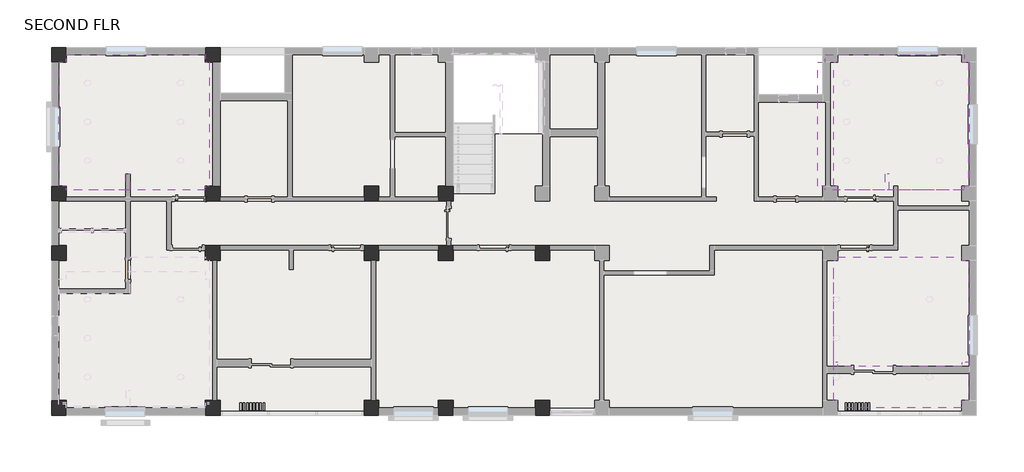
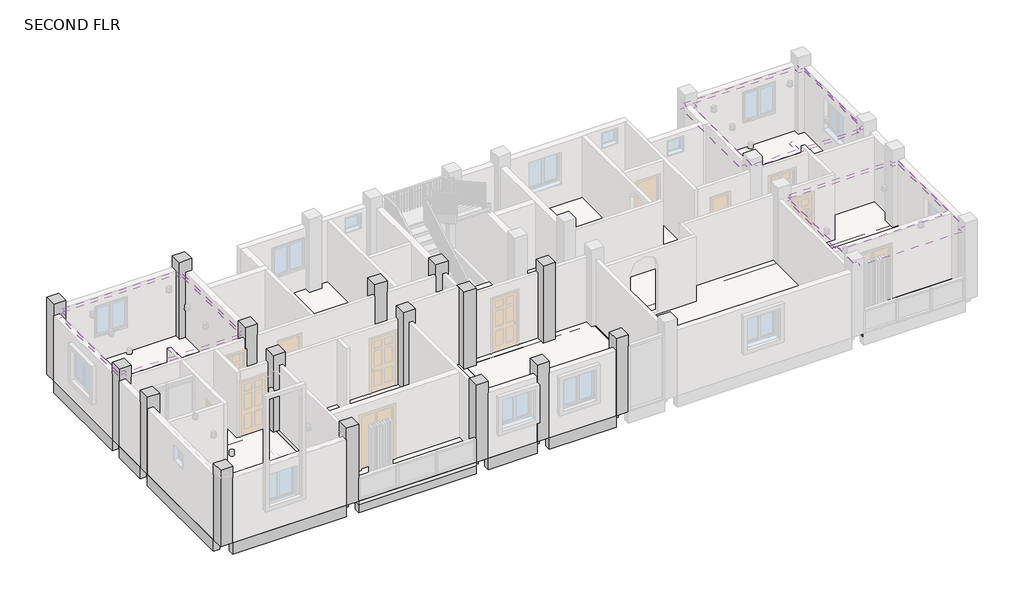
# One storey, part 3 of 5: 23 beams, 16 columns, 6 coverings, 3 slabs.
"""IFC4 building model written with IfcOpenShell, lengths in millimetres."""

from ifc_helpers import new_model, si_unit, point, frame, frame_2d, origin, place, context, project, spatial, polyline, circle_curve, trimmed, segment, composite_curve, outline, extrude, element, save

model = new_model("IFC4")

# Units and contexts
model_context = context("Model", 3, world=origin())
ifc_project = project(units=[si_unit("LENGTHUNIT", "METRE", prefix="MILLI")], contexts=[model_context])

# Site, building, storey
site = spatial("IfcSite", under=ifc_project)
building = spatial("IfcBuilding", under=site)
storey = spatial("IfcBuildingStorey", under=building, Name="SECOND FLR", Elevation=6400.8)

# Beams
placement = place(None, origin())
element("IfcBeam", 1, ObjectType="Concrete-Rectangular Beam : 9\" X 18\" BEAM", at=placement, inside=storey, context=model_context, shape_type="SweptSolid", body=[
    extrude(outline(polyline([(-10649.5456086, -10887.8679047), (-10649.5456086, -11116.4679047), (-14916.7456086, -11116.4679047), (-14916.7456086, -10887.8679047), (-10649.5456086, -10887.8679047)])), frame((0.0, 0.0, 5943.6), z_axis=(0.0, 0.0, 1.0), x_axis=(1.0, 0.0, 0.0)), (0.0, 0.0, 1.0), 457.2),
])
element("IfcBeam", 2, ObjectType="Concrete-Rectangular Beam : 9\" X 18\" BEAM", at=placement, inside=storey, context=model_context, shape_type="SweptSolid", body=[
    extrude(outline(polyline([(-5772.7456086, -10887.8679047), (-5772.7456086, -11116.4679047), (-10192.3456086, -11116.4679047), (-10192.3456086, -10887.8679047), (-5772.7456086, -10887.8679047)])), frame((0.0, 0.0, 5943.6), z_axis=(0.0, 0.0, 1.0), x_axis=(1.0, 0.0, 0.0)), (0.0, 0.0, 1.0), 457.2),
])
element("IfcBeam", 3, ObjectType="Concrete-Rectangular Beam : 9\" X 18\" BEAM", at=placement, inside=storey, context=model_context, shape_type="SweptSolid", body=[
    extrude(outline(polyline([(-3486.7456086, -10887.8679047), (-3486.7456086, -11116.4679047), (-5315.5456086, -11116.4679047), (-5315.5456086, -10887.8679047), (-3486.7456086, -10887.8679047)])), frame((0.0, 0.0, 5943.6), z_axis=(0.0, 0.0, 1.0), x_axis=(1.0, 0.0, 0.0)), (0.0, 0.0, 1.0), 457.2),
])
element("IfcBeam", 4, ObjectType="Concrete-Rectangular Beam : 9\" X 18\" BEAM", at=placement, inside=storey, context=model_context, shape_type="SweptSolid", body=[
    extrude(outline(polyline([(-518.4083398, -10887.8679047), (-518.4083398, -11116.4679047), (-3029.5456086, -11116.4679047), (-3029.5456086, -10887.8679047), (-518.4083398, -10887.8679047)])), frame((0.0, 0.0, 5943.6), z_axis=(0.0, 0.0, 1.0), x_axis=(1.0, 0.0, 0.0)), (0.0, 0.0, 1.0), 457.2),
])
element("IfcBeam", 5, ObjectType="Concrete-Rectangular Beam : 9\" X 18\" BEAM", at=placement, inside=storey, context=model_context, shape_type="SweptSolid", body=[
    extrude(outline(polyline([(-15145.3456086, -4072.3794704), (-15373.9456086, -4072.3794704), (-15373.9456086, -262.3794704), (-15145.3456086, -262.3794704), (-15145.3456086, -4072.3794704)])), frame((0.0, 0.0, 5943.6), z_axis=(0.0, 0.0, 1.0), x_axis=(1.0, 0.0, 0.0)), (0.0, 0.0, 1.0), 457.2),
])
element("IfcBeam", 6, ObjectType="Concrete-Rectangular Beam : 9\" X 18\" BEAM", at=placement, inside=storey, context=model_context, shape_type="SweptSolid", body=[
    extrude(outline(polyline([(-15145.3456086, -5901.1794704), (-15373.9456086, -5901.1794704), (-15373.9456086, -4529.5794704), (-15145.3456086, -4529.5794704), (-15145.3456086, -5901.1794704)])), frame((0.0, 0.0, 5943.6), z_axis=(0.0, 0.0, 1.0), x_axis=(1.0, 0.0, 0.0)), (0.0, 0.0, 1.0), 457.2),
])
element("IfcBeam", 7, ObjectType="Concrete-Rectangular Beam : 9\" X 18\" BEAM", at=placement, inside=storey, context=model_context, shape_type="SweptSolid", body=[
    extrude(outline(polyline([(-15145.3456086, -10659.2679047), (-15373.9456086, -10659.2679047), (-15373.9456086, -6358.3794704), (-15145.3456086, -6358.3794704), (-15145.3456086, -10659.2679047)])), frame((0.0, 0.0, 5943.6), z_axis=(0.0, 0.0, 1.0), x_axis=(1.0, 0.0, 0.0)), (0.0, 0.0, 1.0), 457.2),
])
element("IfcBeam", 8, ObjectType="Concrete-Rectangular Beam : 9\" X 18\" BEAM", at=placement, inside=storey, context=model_context, shape_type="SweptSolid", body=[
    extrude(outline(polyline([(-10649.5456086, -4186.6794704), (-10649.5456086, -4415.2794704), (-14916.7456086, -4415.2794704), (-14916.7456086, -4186.6794704), (-10649.5456086, -4186.6794704)])), frame((0.0, 0.0, 5943.6), z_axis=(0.0, 0.0, 1.0), x_axis=(1.0, 0.0, 0.0)), (0.0, 0.0, 1.0), 457.2),
])
element("IfcBeam", 9, ObjectType="Concrete-Rectangular Beam : 9\" X 18\" BEAM", at=placement, inside=storey, context=model_context, shape_type="SweptSolid", body=[
    extrude(outline(polyline([(-5772.7456086, -4186.6794704), (-5772.7456086, -4415.2794704), (-10192.3456086, -4415.2794704), (-10192.3456086, -4186.6794704), (-5772.7456086, -4186.6794704)])), frame((0.0, 0.0, 5943.6), z_axis=(0.0, 0.0, 1.0), x_axis=(1.0, 0.0, 0.0)), (0.0, 0.0, 1.0), 457.2),
])
element("IfcBeam", 10, ObjectType="Concrete-Rectangular Beam : 9\" X 18\" BEAM", at=placement, inside=storey, context=model_context, shape_type="SweptSolid", body=[
    extrude(outline(polyline([(-3486.7456086, -4186.6794704), (-3486.7456086, -4415.2794704), (-5315.5456086, -4415.2794704), (-5315.5456086, -4186.6794704), (-3486.7456086, -4186.6794704)])), frame((0.0, 0.0, 5943.6), z_axis=(0.0, 0.0, 1.0), x_axis=(1.0, 0.0, 0.0)), (0.0, 0.0, 1.0), 457.2),
])
element("IfcBeam", 11, ObjectType="Concrete-Rectangular Beam : 9\" X 18\" BEAM", at=placement, inside=storey, context=model_context, shape_type="SweptSolid", body=[
    extrude(outline(polyline([(-10306.6456086, -4072.3794704), (-10535.2456086, -4072.3794704), (-10535.2456086, -262.3794704), (-10306.6456086, -262.3794704), (-10306.6456086, -4072.3794704)])), frame((0.0, 0.0, 5943.6), z_axis=(0.0, 0.0, 1.0), x_axis=(1.0, 0.0, 0.0)), (0.0, 0.0, 1.0), 457.2),
])
element("IfcBeam", 12, ObjectType="Concrete-Rectangular Beam : 9\" X 18\" BEAM", at=placement, inside=storey, context=model_context, shape_type="SweptSolid", body=[
    extrude(outline(polyline([(-10649.5456086, -6015.4794704), (-10649.5456086, -6244.0794704), (-14916.7456086, -6244.0794704), (-14916.7456086, -6015.4794704), (-10649.5456086, -6015.4794704)])), frame((0.0, 0.0, 5943.6), z_axis=(0.0, 0.0, 1.0), x_axis=(1.0, 0.0, 0.0)), (0.0, 0.0, 1.0), 457.2),
])
element("IfcBeam", 13, ObjectType="Concrete-Rectangular Beam : 9\" X 18\" BEAM", at=placement, inside=storey, context=model_context, shape_type="SweptSolid", body=[
    extrude(outline(polyline([(-5772.7456086, -6015.4794704), (-5772.7456086, -6244.0794704), (-10192.3456086, -6244.0794704), (-10192.3456086, -6015.4794704), (-5772.7456086, -6015.4794704)])), frame((0.0, 0.0, 5943.6), z_axis=(0.0, 0.0, 1.0), x_axis=(1.0, 0.0, 0.0)), (0.0, 0.0, 1.0), 457.2),
])
element("IfcBeam", 14, ObjectType="Concrete-Rectangular Beam : 9\" X 18\" BEAM", at=placement, inside=storey, context=model_context, shape_type="SweptSolid", body=[
    extrude(outline(polyline([(-3486.7456086, -6015.4794704), (-3486.7456086, -6244.0794704), (-5315.5456086, -6244.0794704), (-5315.5456086, -6015.4794704), (-3486.7456086, -6015.4794704)])), frame((0.0, 0.0, 5943.6), z_axis=(0.0, 0.0, 1.0), x_axis=(1.0, 0.0, 0.0)), (0.0, 0.0, 1.0), 457.2),
])
element("IfcBeam", 15, ObjectType="Concrete-Rectangular Beam : 9\" X 18\" BEAM", at=placement, inside=storey, context=model_context, shape_type="SweptSolid", body=[
    extrude(outline(polyline([(-3029.5456086, -6244.0794704), (-3029.5456086, -6015.4794704), (-518.4083398, -6015.4794704), (-518.4083398, -6244.0794704), (-3029.5456086, -6244.0794704)])), frame((0.0, 0.0, 5943.6), z_axis=(0.0, 0.0, 1.0), x_axis=(1.0, 0.0, 0.0)), (0.0, 0.0, 1.0), 457.2),
])
element("IfcBeam", 16, ObjectType="Concrete-Rectangular Beam : 9\" X 18\" BEAM", at=placement, inside=storey, context=model_context, shape_type="SweptSolid", body=[
    extrude(outline(polyline([(-10535.2456086, -6358.3794704), (-10306.6456086, -6358.3794704), (-10306.6456086, -10659.2679047), (-10535.2456086, -10659.2679047), (-10535.2456086, -6358.3794704)])), frame((0.0, 0.0, 5943.6), z_axis=(0.0, 0.0, 1.0), x_axis=(1.0, 0.0, 0.0)), (0.0, 0.0, 1.0), 457.2),
])
element("IfcBeam", 17, ObjectType="Concrete-Rectangular Beam : 9\" X 18\" BEAM", at=placement, inside=storey, context=model_context, shape_type="SweptSolid", body=[
    extrude(outline(polyline([(-5658.4456086, -6358.3794704), (-5429.8456086, -6358.3794704), (-5429.8456086, -10659.2679047), (-5658.4456086, -10659.2679047), (-5658.4456086, -6358.3794704)])), frame((0.0, 0.0, 5943.6), z_axis=(0.0, 0.0, 1.0), x_axis=(1.0, 0.0, 0.0)), (0.0, 0.0, 1.0), 457.2),
])
element("IfcBeam", 18, ObjectType="Concrete-Rectangular Beam : 9\" X 18\" BEAM", at=placement, inside=storey, context=model_context, shape_type="SweptSolid", body=[
    extrude(outline(polyline([(-3372.4456086, -6358.3794704), (-3143.8456086, -6358.3794704), (-3143.8456086, -10659.2679047), (-3372.4456086, -10659.2679047), (-3372.4456086, -6358.3794704)])), frame((0.0, 0.0, 5943.6), z_axis=(0.0, 0.0, 1.0), x_axis=(1.0, 0.0, 0.0)), (0.0, 0.0, 1.0), 457.2),
])
element("IfcBeam", 19, ObjectType="Concrete-Rectangular Beam : 9\" X 18\" BEAM", at=placement, inside=storey, context=model_context, shape_type="SweptSolid", body=[
    extrude(outline(polyline([(-404.1083398, -6358.3794704), (-175.5083398, -6358.3794704), (-175.5083398, -10659.2679047), (-404.1083398, -10659.2679047), (-404.1083398, -6358.3794704)])), frame((0.0, 0.0, 5943.6), z_axis=(0.0, 0.0, 1.0), x_axis=(1.0, 0.0, 0.0)), (0.0, 0.0, 1.0), 457.2),
])
element("IfcBeam", 20, ObjectType="Concrete-Rectangular Beam : 9\" X 18\" BEAM", at=placement, inside=storey, context=model_context, shape_type="SweptSolid", body=[
    extrude(outline(polyline([(-404.1083398, -4529.5794704), (-175.5083398, -4529.5794704), (-175.5083398, -5901.1794704), (-404.1083398, -5901.1794704), (-404.1083398, -4529.5794704)])), frame((0.0, 0.0, 5943.6), z_axis=(0.0, 0.0, 1.0), x_axis=(1.0, 0.0, 0.0)), (0.0, 0.0, 1.0), 457.2),
])
element("IfcBeam", 21, ObjectType="Concrete-Rectangular Beam : 9\" X 18\" BEAM", at=placement, inside=storey, context=model_context, shape_type="SweptSolid", body=[
    extrude(outline(polyline([(-3143.8456086, -5901.1794704), (-3372.4456086, -5901.1794704), (-3372.4456086, -4529.5794704), (-3143.8456086, -4529.5794704), (-3143.8456086, -5901.1794704)])), frame((0.0, 0.0, 5943.6), z_axis=(0.0, 0.0, 1.0), x_axis=(1.0, 0.0, 0.0)), (0.0, 0.0, 1.0), 457.2),
])
element("IfcBeam", 22, ObjectType="Concrete-Rectangular Beam : 9\" X 18\" BEAM", at=placement, inside=storey, context=model_context, shape_type="SweptSolid", body=[
    extrude(outline(polyline([(-5429.8456086, -5901.1794704), (-5658.4456086, -5901.1794704), (-5658.4456086, -4529.5794704), (-5429.8456086, -4529.5794704), (-5429.8456086, -5901.1794704)])), frame((0.0, 0.0, 5943.6), z_axis=(0.0, 0.0, 1.0), x_axis=(1.0, 0.0, 0.0)), (0.0, 0.0, 1.0), 457.2),
])
element("IfcBeam", 23, ObjectType="Concrete-Rectangular Beam : 9\" X 18\" BEAM", at=placement, inside=storey, context=model_context, shape_type="SweptSolid", body=[
    extrude(outline(polyline([(-10306.6456086, -5901.1794704), (-10535.2456086, -5901.1794704), (-10535.2456086, -4529.5794704), (-10306.6456086, -4529.5794704), (-10306.6456086, -5901.1794704)])), frame((0.0, 0.0, 5943.6), z_axis=(0.0, 0.0, 1.0), x_axis=(1.0, 0.0, 0.0)), (0.0, 0.0, 1.0), 457.2),
])

# Columns
element("IfcColumn", 24, ObjectType="Concrete-Rectangular-Column : COLUMN 18\" X 18\"", at=placement, inside=storey, context=model_context, shape_type="SweptSolid", body=[
    extrude(outline(polyline([(-14916.7456086, 194.8205296), (-14916.7456086, -262.3794704), (-15373.9456086, -262.3794704), (-15373.9456086, 194.8205296), (-14916.7456086, 194.8205296)])), frame((0.0, 0.0, 6400.8), z_axis=(0.0, 0.0, 1.0), x_axis=(1.0, 0.0, 0.0)), (0.0, 0.0, 1.0), 3048.0),
])
element("IfcColumn", 25, ObjectType="Concrete-Rectangular-Column : COLUMN 18\" X 18\"", at=placement, inside=storey, context=model_context, shape_type="SweptSolid", body=[
    extrude(outline(polyline([(-10192.3456086, 194.8205296), (-10192.3456086, -262.3794704), (-10649.5456086, -262.3794704), (-10649.5456086, 194.8205296), (-10192.3456086, 194.8205296)])), frame((0.0, 0.0, 6400.8), z_axis=(0.0, 0.0, 1.0), x_axis=(1.0, 0.0, 0.0)), (0.0, 0.0, 1.0), 3048.0),
])
element("IfcColumn", 26, ObjectType="Concrete-Rectangular-Column : COLUMN 18\" X 18\"", at=placement, inside=storey, context=model_context, shape_type="SweptSolid", body=[
    extrude(outline(polyline([(-61.2083398, -10659.2679047), (-61.2083398, -11116.4679047), (-518.4083398, -11116.4679047), (-518.4083398, -10659.2679047), (-61.2083398, -10659.2679047)])), frame((0.0, 0.0, 6400.8), z_axis=(0.0, 0.0, 1.0), x_axis=(1.0, 0.0, 0.0)), (0.0, 0.0, 1.0), 3048.0),
])
element("IfcColumn", 27, ObjectType="Concrete-Rectangular-Column : COLUMN 18\" X 18\"", at=placement, inside=storey, context=model_context, shape_type="SweptSolid", body=[
    extrude(outline(polyline([(-3029.5456086, -10659.2679047), (-3029.5456086, -11116.4679047), (-3486.7456086, -11116.4679047), (-3486.7456086, -10659.2679047), (-3029.5456086, -10659.2679047)])), frame((0.0, 0.0, 6400.8), z_axis=(0.0, 0.0, 1.0), x_axis=(1.0, 0.0, 0.0)), (0.0, 0.0, 1.0), 3048.0),
])
element("IfcColumn", 28, ObjectType="Concrete-Rectangular-Column : COLUMN 18\" X 18\"", at=placement, inside=storey, context=model_context, shape_type="SweptSolid", body=[
    extrude(outline(polyline([(-5315.5456086, -10659.2679047), (-5315.5456086, -11116.4679047), (-5772.7456086, -11116.4679047), (-5772.7456086, -10659.2679047), (-5315.5456086, -10659.2679047)])), frame((0.0, 0.0, 6400.8), z_axis=(0.0, 0.0, 1.0), x_axis=(1.0, 0.0, 0.0)), (0.0, 0.0, 1.0), 3048.0),
])
element("IfcColumn", 29, ObjectType="Concrete-Rectangular-Column : COLUMN 18\" X 18\"", at=placement, inside=storey, context=model_context, shape_type="SweptSolid", body=[
    extrude(outline(polyline([(-10192.3456086, -10659.2679047), (-10192.3456086, -11116.4679047), (-10649.5456086, -11116.4679047), (-10649.5456086, -10659.2679047), (-10192.3456086, -10659.2679047)])), frame((0.0, 0.0, 6400.8), z_axis=(0.0, 0.0, 1.0), x_axis=(1.0, 0.0, 0.0)), (0.0, 0.0, 1.0), 3048.0),
])
element("IfcColumn", 30, ObjectType="Concrete-Rectangular-Column : COLUMN 18\" X 18\"", at=placement, inside=storey, context=model_context, shape_type="SweptSolid", body=[
    extrude(outline(polyline([(-14916.7456086, -10659.2679047), (-14916.7456086, -11116.4679047), (-15373.9456086, -11116.4679047), (-15373.9456086, -10659.2679047), (-14916.7456086, -10659.2679047)])), frame((0.0, 0.0, 6400.8), z_axis=(0.0, 0.0, 1.0), x_axis=(1.0, 0.0, 0.0)), (0.0, 0.0, 1.0), 3048.0),
])
element("IfcColumn", 31, ObjectType="Concrete-Rectangular-Column : COLUMN 18\" X 18\"", at=placement, inside=storey, context=model_context, shape_type="SweptSolid", body=[
    extrude(outline(polyline([(-14916.7456086, -5901.1794704), (-14916.7456086, -6358.3794704), (-15373.9456086, -6358.3794704), (-15373.9456086, -5901.1794704), (-14916.7456086, -5901.1794704)])), frame((0.0, 0.0, 6400.8), z_axis=(0.0, 0.0, 1.0), x_axis=(1.0, 0.0, 0.0)), (0.0, 0.0, 1.0), 3048.0),
])
element("IfcColumn", 32, ObjectType="Concrete-Rectangular-Column : COLUMN 18\" X 18\"", at=placement, inside=storey, context=model_context, shape_type="SweptSolid", body=[
    extrude(outline(polyline([(-14916.7456086, -4072.3794704), (-14916.7456086, -4529.5794704), (-15373.9456086, -4529.5794704), (-15373.9456086, -4072.3794704), (-14916.7456086, -4072.3794704)])), frame((0.0, 0.0, 6400.8), z_axis=(0.0, 0.0, 1.0), x_axis=(1.0, 0.0, 0.0)), (0.0, 0.0, 1.0), 3048.0),
])
element("IfcColumn", 33, ObjectType="Concrete-Rectangular-Column : COLUMN 18\" X 18\"", at=placement, inside=storey, context=model_context, shape_type="SweptSolid", body=[
    extrude(outline(polyline([(-10192.3456086, -4072.3794704), (-10192.3456086, -4529.5794704), (-10649.5456086, -4529.5794704), (-10649.5456086, -4072.3794704), (-10192.3456086, -4072.3794704)])), frame((0.0, 0.0, 6400.8), z_axis=(0.0, 0.0, 1.0), x_axis=(1.0, 0.0, 0.0)), (0.0, 0.0, 1.0), 3048.0),
])
element("IfcColumn", 34, ObjectType="Concrete-Rectangular-Column : COLUMN 18\" X 18\"", at=placement, inside=storey, context=model_context, shape_type="SweptSolid", body=[
    extrude(outline(polyline([(-5315.5456086, -4072.3794704), (-5315.5456086, -4529.5794704), (-5772.7456086, -4529.5794704), (-5772.7456086, -4072.3794704), (-5315.5456086, -4072.3794704)])), frame((0.0, 0.0, 6400.8), z_axis=(0.0, 0.0, 1.0), x_axis=(1.0, 0.0, 0.0)), (0.0, 0.0, 1.0), 3048.0),
])
element("IfcColumn", 35, ObjectType="Concrete-Rectangular-Column : COLUMN 18\" X 18\"", at=placement, inside=storey, context=model_context, shape_type="SweptSolid", body=[
    extrude(outline(polyline([(-3029.5456086, -4072.3794704), (-3029.5456086, -4529.5794704), (-3486.7456086, -4529.5794704), (-3486.7456086, -4072.3794704), (-3029.5456086, -4072.3794704)])), frame((0.0, 0.0, 6400.8), z_axis=(0.0, 0.0, 1.0), x_axis=(1.0, 0.0, 0.0)), (0.0, 0.0, 1.0), 3048.0),
])
element("IfcColumn", 36, ObjectType="Concrete-Rectangular-Column : COLUMN 18\" X 18\"", at=placement, inside=storey, context=model_context, shape_type="SweptSolid", body=[
    extrude(outline(polyline([(-61.2083398, -5901.1794704), (-61.2083398, -6358.3794704), (-518.4083398, -6358.3794704), (-518.4083398, -5901.1794704), (-61.2083398, -5901.1794704)])), frame((0.0, 0.0, 6400.8), z_axis=(0.0, 0.0, 1.0), x_axis=(1.0, 0.0, 0.0)), (0.0, 0.0, 1.0), 3048.0),
])
element("IfcColumn", 37, ObjectType="Concrete-Rectangular-Column : COLUMN 18\" X 18\"", at=placement, inside=storey, context=model_context, shape_type="SweptSolid", body=[
    extrude(outline(polyline([(-3029.5456086, -5901.1794704), (-3029.5456086, -6358.3794704), (-3486.7456086, -6358.3794704), (-3486.7456086, -5901.1794704), (-3029.5456086, -5901.1794704)])), frame((0.0, 0.0, 6400.8), z_axis=(0.0, 0.0, 1.0), x_axis=(1.0, 0.0, 0.0)), (0.0, 0.0, 1.0), 3048.0),
])
element("IfcColumn", 38, ObjectType="Concrete-Rectangular-Column : COLUMN 18\" X 18\"", at=placement, inside=storey, context=model_context, shape_type="SweptSolid", body=[
    extrude(outline(polyline([(-5315.5456086, -5901.1794704), (-5315.5456086, -6358.3794704), (-5772.7456086, -6358.3794704), (-5772.7456086, -5901.1794704), (-5315.5456086, -5901.1794704)])), frame((0.0, 0.0, 6400.8), z_axis=(0.0, 0.0, 1.0), x_axis=(1.0, 0.0, 0.0)), (0.0, 0.0, 1.0), 3048.0),
])
element("IfcColumn", 39, ObjectType="Concrete-Rectangular-Column : COLUMN 18\" X 18\"", at=placement, inside=storey, context=model_context, shape_type="SweptSolid", body=[
    extrude(outline(polyline([(-10192.3456086, -5901.1794704), (-10192.3456086, -6358.3794704), (-10649.5456086, -6358.3794704), (-10649.5456086, -5901.1794704), (-10192.3456086, -5901.1794704)])), frame((0.0, 0.0, 6400.8), z_axis=(0.0, 0.0, 1.0), x_axis=(1.0, 0.0, 0.0)), (0.0, 0.0, 1.0), 3048.0),
])

# Coverings
element("IfcCovering", 40, ObjectType="GWB on Mtl. Stud", at=placement, inside=storey, context=model_context, shape_type="SweptSolid", body=[
    extrude(outline(polyline([(-14916.7456086, -262.3794704), (-14916.7456086, -33.7794704), (-10649.5456086, -33.7794704), (-10649.5456086, -262.3794704), (-10535.2456086, -262.3794704), (-10535.2456086, -4072.3794704), (-10649.5456086, -4072.3794704), (-10649.5456086, -4186.6794704), (-12959.7401855, -4186.6794704), (-12959.7401855, -3705.5659448), (-13086.7401855, -3705.5659448), (-13086.7401855, -4186.6794704), (-14916.7456086, -4186.6794704), (-14916.7456086, -4072.3794704), (-15145.3456086, -4072.3794704), (-15145.3456086, -262.3794704), (-14916.7456086, -262.3794704)]), holes=[composite_curve([segment(trimmed(circle_curve(frame_2d((-14269.0456086, -897.3794704)), 76.2), [point((-14345.2456086, -897.3794704))], [point((-14192.8456086, -897.3794704))], True, "CARTESIAN"), True, "CONTINUOUS"), segment(trimmed(circle_curve(frame_2d((-14269.0456086, -897.3794704)), 76.2), [point((-14192.8456086, -897.3794704))], [point((-14345.2456086, -897.3794704))], True, "CARTESIAN"), True, "CONTINUOUS")], self_intersect=False), composite_curve([segment(trimmed(circle_curve(frame_2d((-14269.0456086, -3284.9794704)), 76.2), [point((-14345.2456086, -3284.9794704))], [point((-14192.8456086, -3284.9794704))], True, "CARTESIAN"), True, "CONTINUOUS"), segment(trimmed(circle_curve(frame_2d((-14269.0456086, -3284.9794704)), 76.2), [point((-14192.8456086, -3284.9794704))], [point((-14345.2456086, -3284.9794704))], True, "CARTESIAN"), True, "CONTINUOUS")], self_intersect=False), composite_curve([segment(trimmed(circle_curve(frame_2d((-14269.0456086, -2091.1794704)), 76.2), [point((-14345.2456086, -2091.1794704))], [point((-14192.8456086, -2091.1794704))], True, "CARTESIAN"), True, "CONTINUOUS"), segment(trimmed(circle_curve(frame_2d((-14269.0456086, -2091.1794704)), 76.2), [point((-14192.8456086, -2091.1794704))], [point((-14345.2456086, -2091.1794704))], True, "CARTESIAN"), True, "CONTINUOUS")], self_intersect=False), composite_curve([segment(trimmed(circle_curve(frame_2d((-11411.5456086, -897.3794704)), 76.2), [point((-11335.3456086, -897.3794704))], [point((-11487.7456086, -897.3794704))], True, "CARTESIAN"), True, "CONTINUOUS"), segment(trimmed(circle_curve(frame_2d((-11411.5456086, -897.3794704)), 76.2), [point((-11487.7456086, -897.3794704))], [point((-11335.3456086, -897.3794704))], True, "CARTESIAN"), True, "CONTINUOUS")], self_intersect=False), composite_curve([segment(trimmed(circle_curve(frame_2d((-11411.5456086, -3284.9794704)), 76.2), [point((-11335.3456086, -3284.9794704))], [point((-11487.7456086, -3284.9794704))], True, "CARTESIAN"), True, "CONTINUOUS"), segment(trimmed(circle_curve(frame_2d((-11411.5456086, -3284.9794704)), 76.2), [point((-11487.7456086, -3284.9794704))], [point((-11335.3456086, -3284.9794704))], True, "CARTESIAN"), True, "CONTINUOUS")], self_intersect=False), composite_curve([segment(trimmed(circle_curve(frame_2d((-11411.5456086, -2091.1794704)), 76.2), [point((-11335.3456086, -2091.1794704))], [point((-11487.7456086, -2091.1794704))], True, "CARTESIAN"), True, "CONTINUOUS"), segment(trimmed(circle_curve(frame_2d((-11411.5456086, -2091.1794704)), 76.2), [point((-11487.7456086, -2091.1794704))], [point((-11335.3456086, -2091.1794704))], True, "CARTESIAN"), True, "CONTINUOUS")], self_intersect=False)]), frame((0.0, 0.0, 8966.2), z_axis=(0.0, 0.0, 1.0), x_axis=(1.0, 0.0, 0.0)), (0.0, 0.0, 1.0), 107.95),
])
element("IfcCovering", 41, ObjectType="GWB on Mtl. Stud", at=placement, inside=storey, context=model_context, shape_type="SweptSolid", body=[
    extrude(outline(polyline([(-15145.3456086, -4072.3794704), (-15145.3456086, -262.3794704), (-14916.7456086, -262.3794704), (-14916.7456086, -33.7794704), (-10649.5456086, -33.7794704), (-10649.5456086, -262.3794704), (-10535.2456086, -262.3794704), (-10535.2456086, -4072.3794704), (-10649.5456086, -4072.3794704), (-10649.5456086, -4186.6794704), (-12959.7401855, -4186.6794704), (-14916.7456086, -4186.6794704), (-14916.7456086, -4072.3794704), (-15145.3456086, -4072.3794704)]), holes=[polyline([(-14840.5456086, -3881.8794704), (-10840.0456086, -3881.8794704), (-10840.0456086, -338.5794704), (-14840.5456086, -338.5794704), (-14840.5456086, -3881.8794704)])]), frame((0.0, 0.0, 8839.2), z_axis=(0.0, 0.0, 1.0), x_axis=(1.0, 0.0, 0.0)), (0.0, 0.0, 1.0), 107.95),
    extrude(outline(polyline([(-14688.1456086, -3729.4794704), (-14688.1456086, -490.9794704), (-10992.4456086, -490.9794704), (-10992.4456086, -3729.4794704), (-14688.1456086, -3729.4794704)]), holes=[polyline([(-11144.8456086, -643.3794704), (-14535.7456086, -643.3794704), (-14535.7456086, -3577.0794704), (-11144.8456086, -3577.0794704), (-11144.8456086, -643.3794704)])]), frame((0.0, 0.0, 8839.2), z_axis=(0.0, 0.0, 1.0), x_axis=(1.0, 0.0, 0.0)), (0.0, 0.0, 1.0), 107.95),
])
element("IfcCovering", 42, ObjectType="GWB on Mtl. Stud", at=placement, inside=storey, context=model_context, shape_type="SweptSolid", body=[
    extrude(outline(polyline([(8991.0043914, -3729.4794704), (8991.0043914, -490.9794704), (12477.1543914, -490.9794704), (12477.1543914, -3729.4794704), (8991.0043914, -3729.4794704)]), holes=[polyline([(12324.7543914, -643.3794704), (9162.4543914, -643.3794704), (9162.4543914, -3577.0794704), (12324.7543914, -3577.0794704), (12324.7543914, -643.3794704)])]), frame((0.0, 0.0, 8839.2), z_axis=(0.0, 0.0, 1.0), x_axis=(1.0, 0.0, 0.0)), (0.0, 0.0, 1.0), 107.95),
    extrude(outline(polyline([(8660.1098601, -4072.3794704), (8660.1098601, -262.3794704), (8774.4128058, -262.3794704), (8774.4128058, -33.7794704), (12584.4128058, -33.7794704), (12584.4128058, -262.3794704), (12813.0098601, -262.3794704), (12813.0098601, -4072.3794704), (12584.4128058, -4072.3794704), (12584.4128058, -4186.6794704), (10509.8598145, -4186.6794704), (8774.4128058, -4186.6794704), (8774.4128058, -4072.3794704), (8660.1098601, -4072.3794704)]), holes=[polyline([(8838.6043914, -338.5794704), (8838.6043914, -3881.8794704), (12629.5543914, -3881.8794704), (12629.5543914, -338.5794704), (8838.6043914, -338.5794704)])]), frame((0.0, 0.0, 8839.2), z_axis=(0.0, 0.0, 1.0), x_axis=(1.0, 0.0, 0.0)), (0.0, 0.0, 1.0), 107.95),
])
element("IfcCovering", 43, ObjectType="GWB on Mtl. Stud", at=placement, inside=storey, context=model_context, shape_type="SweptSolid", body=[
    extrude(outline(polyline([(8991.0043914, -9147.9642361), (8991.0043914, -6726.6794704), (12477.1543914, -6726.6794704), (12477.1543914, -9147.9642361), (8991.0043914, -9147.9642361)]), holes=[polyline([(12324.7543914, -7031.4298611), (9162.4543914, -7031.4298611), (9162.4543914, -8995.5642361), (12324.7543914, -8995.5642361), (12324.7543914, -7031.4298611)])]), frame((0.0, 0.0, 8839.2), z_axis=(0.0, 0.0, 1.0), x_axis=(1.0, 0.0, 0.0)), (0.0, 0.0, 1.0), 107.95),
    extrude(outline(polyline([(8660.1098601, -9490.8642361), (8660.1098601, -6358.3685356), (8774.4128058, -6358.3685356), (8774.4128058, -6244.0794704), (12584.4128058, -6244.0794704), (12584.4128058, -6358.3794704), (12813.0098601, -6358.3794704), (12813.0098601, -9490.8642361), (12584.4128058, -9490.8642361), (12584.4128058, -9605.1642361), (10509.8598145, -9605.1642361), (8774.4128058, -9605.1642361), (8774.4128058, -9490.8642361), (8660.1098601, -9490.8642361)]), holes=[polyline([(12629.5543914, -6498.0794704), (8838.6043914, -6498.0794704), (8838.6043914, -9300.3642361), (12629.5543914, -9300.3642361), (12629.5543914, -6498.0794704)])]), frame((0.0, 0.0, 8839.2), z_axis=(0.0, 0.0, 1.0), x_axis=(1.0, 0.0, 0.0)), (0.0, 0.0, 1.0), 107.95),
])
element("IfcCovering", 44, ObjectType="GWB on Mtl. Stud", at=placement, inside=storey, context=model_context, shape_type="SweptSolid", body=[
    extrude(outline(polyline([(8400.4543914, -262.3794704), (8400.4543914, -33.7794704), (12667.6543914, -33.7794704), (12667.6543914, -262.3794704), (12781.9543914, -262.3794704), (12781.9543914, -4072.3794704), (12667.6543914, -4072.3794704), (12667.6543914, -4186.6794704), (10357.4598145, -4186.6794704), (10357.4598145, -3705.5659448), (10230.4598145, -3705.5659448), (10230.4598145, -4186.6794704), (8400.4543914, -4186.6794704), (8400.4543914, -4072.3794704), (8171.8543914, -4072.3794704), (8171.8543914, -262.3794704), (8400.4543914, -262.3794704)]), holes=[composite_curve([segment(trimmed(circle_curve(frame_2d((9048.1543914, -897.3794704)), 76.2), [point((8971.9543914, -897.3794704))], [point((9124.3543914, -897.3794704))], True, "CARTESIAN"), True, "CONTINUOUS"), segment(trimmed(circle_curve(frame_2d((9048.1543914, -897.3794704)), 76.2), [point((9124.3543914, -897.3794704))], [point((8971.9543914, -897.3794704))], True, "CARTESIAN"), True, "CONTINUOUS")], self_intersect=False), composite_curve([segment(trimmed(circle_curve(frame_2d((9048.1543914, -3284.9794704)), 76.2), [point((8971.9543914, -3284.9794704))], [point((9124.3543914, -3284.9794704))], True, "CARTESIAN"), True, "CONTINUOUS"), segment(trimmed(circle_curve(frame_2d((9048.1543914, -3284.9794704)), 76.2), [point((9124.3543914, -3284.9794704))], [point((8971.9543914, -3284.9794704))], True, "CARTESIAN"), True, "CONTINUOUS")], self_intersect=False), composite_curve([segment(trimmed(circle_curve(frame_2d((9048.1543914, -2091.1794704)), 76.2), [point((8971.9543914, -2091.1794704))], [point((9124.3543914, -2091.1794704))], True, "CARTESIAN"), True, "CONTINUOUS"), segment(trimmed(circle_curve(frame_2d((9048.1543914, -2091.1794704)), 76.2), [point((9124.3543914, -2091.1794704))], [point((8971.9543914, -2091.1794704))], True, "CARTESIAN"), True, "CONTINUOUS")], self_intersect=False), composite_curve([segment(trimmed(circle_curve(frame_2d((11905.6543914, -897.3794704)), 76.2), [point((11981.8543914, -897.3794704))], [point((11829.4543914, -897.3794704))], True, "CARTESIAN"), True, "CONTINUOUS"), segment(trimmed(circle_curve(frame_2d((11905.6543914, -897.3794704)), 76.2), [point((11829.4543914, -897.3794704))], [point((11981.8543914, -897.3794704))], True, "CARTESIAN"), True, "CONTINUOUS")], self_intersect=False), composite_curve([segment(trimmed(circle_curve(frame_2d((11905.6543914, -3284.9794704)), 76.2), [point((11981.8543914, -3284.9794704))], [point((11829.4543914, -3284.9794704))], True, "CARTESIAN"), True, "CONTINUOUS"), segment(trimmed(circle_curve(frame_2d((11905.6543914, -3284.9794704)), 76.2), [point((11829.4543914, -3284.9794704))], [point((11981.8543914, -3284.9794704))], True, "CARTESIAN"), True, "CONTINUOUS")], self_intersect=False)]), frame((0.0, 0.0, 8966.2), z_axis=(0.0, 0.0, 1.0), x_axis=(1.0, 0.0, 0.0)), (0.0, 0.0, 1.0), 107.95),
])
element("IfcCovering", 45, ObjectType="GWB on Mtl. Stud", at=placement, inside=storey, context=model_context, shape_type="SweptSolid", body=[
    extrude(outline(polyline([(8660.8043914, -6917.1794704), (8660.8043914, -6358.3794704), (8774.4128058, -6358.3794704), (8774.4128058, -6244.0794704), (12584.4128058, -6244.0794704), (12584.4128058, -6358.3794704), (12813.0098601, -6358.3794704), (12813.0098601, -10659.2679047), (12584.4128058, -10659.2679047), (12584.4128058, -10887.8673366), (8774.4128058, -10887.8673366), (8774.4128058, -10659.2679047), (8660.8043914, -10659.2679047), (8660.8043914, -6917.1794704)]), holes=[composite_curve([segment(trimmed(circle_curve(frame_2d((8743.3543914, -7552.1794704)), 76.2), [point((8667.1543914, -7552.1794704))], [point((8819.5543914, -7552.1794704))], True, "CARTESIAN"), True, "CONTINUOUS"), segment(trimmed(circle_curve(frame_2d((8743.3543914, -7552.1794704)), 76.2), [point((8819.5543914, -7552.1794704))], [point((8667.1543914, -7552.1794704))], True, "CARTESIAN"), True, "CONTINUOUS")], self_intersect=False), composite_curve([segment(trimmed(circle_curve(frame_2d((8743.3543914, -9939.7794704)), 76.2), [point((8667.1543914, -9939.7794704))], [point((8819.5543914, -9939.7794704))], True, "CARTESIAN"), True, "CONTINUOUS"), segment(trimmed(circle_curve(frame_2d((8743.3543914, -9939.7794704)), 76.2), [point((8819.5543914, -9939.7794704))], [point((8667.1543914, -9939.7794704))], True, "CARTESIAN"), True, "CONTINUOUS")], self_intersect=False), composite_curve([segment(trimmed(circle_curve(frame_2d((8743.3543914, -8745.9794704)), 76.2), [point((8667.1543914, -8745.9794704))], [point((8819.5543914, -8745.9794704))], True, "CARTESIAN"), True, "CONTINUOUS"), segment(trimmed(circle_curve(frame_2d((8743.3543914, -8745.9794704)), 76.2), [point((8819.5543914, -8745.9794704))], [point((8667.1543914, -8745.9794704))], True, "CARTESIAN"), True, "CONTINUOUS")], self_intersect=False), composite_curve([segment(trimmed(circle_curve(frame_2d((11600.8543914, -7552.1794704)), 76.2), [point((11677.0543914, -7552.1794704))], [point((11524.6543914, -7552.1794704))], True, "CARTESIAN"), True, "CONTINUOUS"), segment(trimmed(circle_curve(frame_2d((11600.8543914, -7552.1794704)), 76.2), [point((11524.6543914, -7552.1794704))], [point((11677.0543914, -7552.1794704))], True, "CARTESIAN"), True, "CONTINUOUS")], self_intersect=False), composite_curve([segment(trimmed(circle_curve(frame_2d((11600.8543914, -9939.7794704)), 76.2), [point((11677.0543914, -9939.7794704))], [point((11524.6543914, -9939.7794704))], True, "CARTESIAN"), True, "CONTINUOUS"), segment(trimmed(circle_curve(frame_2d((11600.8543914, -9939.7794704)), 76.2), [point((11524.6543914, -9939.7794704))], [point((11677.0543914, -9939.7794704))], True, "CARTESIAN"), True, "CONTINUOUS")], self_intersect=False)]), frame((0.0, 0.0, 8966.2), z_axis=(0.0, 0.0, 1.0), x_axis=(1.0, 0.0, 0.0)), (0.0, 0.0, 1.0), 107.95),
])

# Slabs
element("IfcSlab", 46, ObjectType="white MARBLE FLOORING 6\" 2", at=placement, inside=storey, context=model_context, shape_type="SweptSolid", body=[
    extrude(outline(polyline([(-14916.7456086, -262.3794704), (-14916.7456086, -33.7794704), (-10649.5456086, -33.7794704), (-10649.5456086, -262.3794704), (-10420.9456086, -262.3794704), (-10420.9456086, -4072.3794704), (-10649.5456086, -4072.3794704), (-10649.5456086, -4529.5794704), (-11614.7456086, -4529.5794704), (-11614.7456086, -4402.5794704), (-12959.7401855, -4402.5794704), (-12959.7401855, -3705.5659448), (-13086.7401855, -3705.5659448), (-13086.7401855, -4402.5794704), (-14916.7456086, -4402.5794704), (-14916.7456086, -4072.3794704), (-15145.3456086, -4072.3794704), (-15145.3456086, -262.3794704), (-14916.7456086, -262.3794704)])), frame((0.0, 0.0, 6248.4), z_axis=(0.0, 0.0, 1.0), x_axis=(1.0, 0.0, 0.0)), (0.0, 0.0, 1.0), 152.4),
    extrude(outline(polyline([(-15145.3456086, -7363.1659448), (-12959.7401855, -7363.1659448), (-12959.7401855, -4529.5794704), (-11829.4401855, -4529.5794704), (-11829.4401855, -6028.1794704), (-10649.5456086, -6028.1794704), (-10649.5456086, -6358.3794704), (-10420.9456086, -6358.3794704), (-10420.9456086, -10659.2679047), (-10649.5456086, -10659.2679047), (-10649.5456086, -10887.8679047), (-14916.7456086, -10887.8679047), (-14916.7456086, -10659.2679047), (-15145.3456086, -10659.2679047), (-15145.3456086, -7363.1659448)])), frame((0.0, 0.0, 6248.4), z_axis=(0.0, 0.0, 1.0), x_axis=(1.0, 0.0, 0.0)), (0.0, 0.0, 1.0), 152.4),
    extrude(outline(polyline([(-5772.7456086, -11116.4679047), (-10192.3456086, -11116.4679047), (-10192.3456086, -10659.2679047), (-10293.9456086, -10659.2679047), (-10293.9456086, -9630.5679047), (-9239.8456086, -9630.5679047), (-9239.8456086, -9401.9679047), (-10293.9456086, -9401.9679047), (-10293.9456086, -6358.3794704), (-10192.3456086, -6358.3794704), (-10192.3456086, -6028.1794704), (-8071.4456086, -6028.1794704), (-8071.4456086, -6637.7794704), (-7944.4456086, -6637.7794704), (-7944.4456086, -6028.1794704), (-6788.7456086, -6028.1794704), (-6788.7456086, -5901.1794704), (-5874.3456086, -5901.1794704), (-5874.3456086, -6028.1794704), (-5772.7456086, -6028.1794704), (-5772.7456086, -6358.3794704), (-5544.1456086, -6358.3794704), (-5544.1456086, -9401.9679047), (-8020.6456086, -9401.9679047), (-8020.6456086, -9630.5679047), (-5544.1456086, -9630.5679047), (-5544.1456086, -10659.2679047), (-5772.7456086, -10659.2679047), (-5772.7456086, -11116.4679047)])), frame((0.0, 0.0, 6248.4), z_axis=(0.0, 0.0, 1.0), x_axis=(1.0, 0.0, 0.0)), (0.0, 0.0, 1.0), 152.4),
    extrude(outline(polyline([(-5315.5456086, -10659.2679047), (-5417.1456086, -10659.2679047), (-5417.1456086, -6358.3794704), (-5315.5456086, -6358.3794704), (-5315.5456086, -6028.1794704), (-3486.7456086, -6028.1794704), (-3486.7456086, -6358.3794704), (-3029.5456086, -6358.3794704), (-3029.5456086, -6028.1794704), (-2231.1769742, -6028.1794704), (-2231.1769742, -5901.1794704), (-1316.7769742, -5901.1794704), (-1316.7769742, -6028.1794704), (-518.4083398, -6028.1794704), (-518.4083398, -6358.3794704), (-61.2083398, -6358.3794704), (-61.2083398, -6028.1794704), (1310.3916602, -6028.1794704), (1310.3916602, -6358.3794704), (1462.7916602, -6358.3794704), (1462.7916602, -10659.2679047), (1310.3916602, -10659.2679047), (1310.3916602, -10887.8679047), (-61.2083398, -10887.8679047), (-61.2083398, -10659.2679047), (-518.4083398, -10659.2679047), (-518.4083398, -10887.8679047), (-3029.5456086, -10887.8679047), (-3029.5456086, -10659.2679047), (-3486.7456086, -10659.2679047), (-3486.7456086, -10887.8679047), (-5315.5456086, -10887.8679047), (-5315.5456086, -10659.2679047)])), frame((0.0, 0.0, 6248.4), z_axis=(0.0, 0.0, 1.0), x_axis=(1.0, 0.0, 0.0)), (0.0, 0.0, 1.0), 152.4),
    extrude(outline(polyline([(1589.7916602, -6802.8794704), (4980.6916602, -6802.8794704), (4980.6916602, -6028.1794704), (8317.2128058, -6028.1794704), (8317.2128058, -10887.8679047), (1767.5916602, -10887.8679047), (1767.5916602, -10659.2679047), (1589.7916602, -10659.2679047), (1589.7916602, -6802.8794704)])), frame((0.0, 0.0, 6248.4), z_axis=(0.0, 0.0, 1.0), x_axis=(1.0, 0.0, 0.0)), (0.0, 0.0, 1.0), 152.4),
    extrude(outline(polyline([(8774.4128058, -10659.2679047), (8444.2128058, -10659.2679047), (8444.2128058, -9833.7679047), (9269.7128058, -9833.7679047), (9269.7128058, -9605.1679047), (8444.2128058, -9605.1679047), (8444.2128058, -6358.3794704), (8774.4128058, -6358.3794704), (8774.4128058, -6028.1794704), (8850.6128058, -6028.1794704), (8850.6128058, -5901.1794704), (9765.0128058, -5901.1794704), (9765.0128058, -6028.1794704), (9790.4128058, -6028.1794704), (10628.6128058, -6028.1794704), (10628.6128058, -4808.9794704), (12813.0128058, -4808.9794704), (12813.0128058, -5901.1794704), (12584.4128058, -5901.1794704), (12584.4128058, -6358.3794704), (12813.0128058, -6358.3794704), (12813.0128058, -9605.1679047), (10488.9128058, -9605.1679047), (10488.9128058, -9833.7679047), (12813.0128058, -9833.7679047), (12813.0128058, -10659.2679047), (12584.4128058, -10659.2679047), (12584.4128058, -11052.9679047), (8774.4128058, -11052.9679047), (8774.4128058, -10659.2679047)])), frame((0.0, 0.0, 6248.4), z_axis=(0.0, 0.0, 1.0), x_axis=(1.0, 0.0, 0.0)), (0.0, 0.0, 1.0), 152.4),
    extrude(outline(polyline([(9968.2128058, -4529.5794704), (9053.8128058, -4529.5794704), (8774.4128058, -4529.5794704), (8774.4128058, -4072.3794704), (8545.8128058, -4072.3794704), (8545.8128058, -262.3794704), (8774.4128058, -262.3794704), (8774.4128058, -33.7794704), (12584.4128058, -33.7794704), (12584.4128058, -262.3794704), (12813.0128058, -262.3794704), (12813.0128058, -4072.3794704), (12584.4128058, -4072.3794704), (12584.4128058, -4529.5794704), (12813.0128058, -4529.5794704), (12813.0128058, -4681.9794704), (10628.6128058, -4681.9794704), (10628.6128058, -4072.3794704), (10501.6128058, -4072.3794704), (10501.6128058, -4402.5794704), (9968.2128058, -4402.5794704), (9968.2128058, -4529.5794704)])), frame((0.0, 0.0, 6248.4), z_axis=(0.0, 0.0, 1.0), x_axis=(1.0, 0.0, 0.0)), (0.0, 0.0, 1.0), 152.4),
])
element("IfcSlab", 47, ObjectType="white MARBLE FLOORING 6\" 2", at=placement, inside=storey, context=model_context, shape_type="SweptSolid", body=[
    extrude(outline(polyline([(-11702.4401855, -5901.1794704), (-11702.4401855, -4529.5794704), (-8604.8456086, -4529.5794704), (-3232.7456086, -4529.5794704), (-3232.7456086, -4758.1794704), (-3105.7456086, -4758.1794704), (-3105.7456086, -4529.5794704), (-3029.5456086, -4529.5794704), (-3029.5456086, -4300.9794704), (-1759.5456086, -4300.9794704), (-1759.5456086, -2472.1794704), (-289.8083398, -2472.1794704), (-289.8083398, -4072.3794704), (-518.4083398, -4072.3794704), (-518.4083398, -4529.5794704), (-61.2083398, -4529.5794704), (-61.2083398, -2548.3794704), (1399.2916602, -2548.3794704), (1399.2916602, -4072.3794704), (1310.3916602, -4072.3794704), (1310.3916602, -4529.5794704), (5044.1916602, -4529.5794704), (5044.1916602, -4402.5794704), (4726.6916602, -4402.5794704), (4726.6916602, -2535.6794704), (6212.5916602, -2535.6794704), (6212.5916602, -4529.5794704), (10501.6128058, -4529.5794704), (10501.6128058, -5901.1794704), (4853.6916602, -5901.1794704), (4853.6916602, -6675.8794704), (1589.7916602, -6675.8794704), (1589.7916602, -6358.3794704), (1767.5916602, -6358.3794704), (1767.5916602, -5901.1794704), (-3105.7456086, -5901.1794704), (-3105.7456086, -5672.5794704), (-3232.7456086, -5672.5794704), (-3232.7456086, -5901.1794704), (-10750.542897, -5901.1794704), (-10750.542897, -6028.1794704), (-11664.942897, -6028.1794704), (-11664.942897, -5901.1794704), (-11702.4401855, -5901.1794704)])), frame((0.0, 0.0, 6248.4), z_axis=(0.0, 0.0, 1.0), x_axis=(1.0, 0.0, 0.0)), (0.0, 0.0, 1.0), 152.4),
])
element("IfcSlab", 48, ObjectType="white MARBLE FLOORING 6\" 2", at=placement, inside=storey, context=model_context, shape_type="SweptSolid", body=[
    extrude(outline(polyline([(-61.2083398, -2319.7794704), (-61.2083398, -33.7794704), (1310.3916602, -33.7794704), (1310.3916602, -262.3794704), (1399.2916602, -262.3794704), (1399.2916602, -2319.7794704), (-61.2083398, -2319.7794704)])), frame((0.0, 0.0, 6400.8), z_axis=(0.0, 0.0, 1.0), x_axis=(1.0, 0.0, 0.0)), (0.0, 0.0, 1.0), 152.4),
    extrude(outline(polyline([(1767.5916602, -4072.3794704), (1627.8916602, -4072.3794704), (1627.8916602, -262.3794704), (1767.5916602, -262.3794704), (1767.5916602, -33.7794704), (4599.6916602, -33.7794704), (4599.6916602, -4402.5794704), (1767.5916602, -4402.5794704), (1767.5916602, -4072.3794704)])), frame((0.0, 0.0, 6400.8), z_axis=(0.0, 0.0, 1.0), x_axis=(1.0, 0.0, 0.0)), (0.0, 0.0, 1.0), 152.4),
    extrude(outline(polyline([(6212.5916602, -33.7794704), (6212.5916602, -2408.6794704), (5996.6916602, -2408.6794704), (5996.6916602, -2535.6794704), (5234.6916602, -2535.6794704), (5234.6916602, -2408.6794704), (4726.6916602, -2408.6794704), (4726.6916602, -33.7794704), (6212.5916602, -33.7794704)])), frame((0.0, 0.0, 6400.8), z_axis=(0.0, 0.0, 1.0), x_axis=(1.0, 0.0, 0.0)), (0.0, 0.0, 1.0), 152.4),
    extrude(outline(polyline([(6885.6916602, -4402.5794704), (6339.5916602, -4402.5794704), (6339.5916602, -1481.5794704), (8418.8128058, -1481.5794704), (8418.8128058, -4072.3794704), (8317.2128058, -4072.3794704), (8317.2128058, -4402.5794704), (7495.2916602, -4402.5794704), (7495.2916602, -4529.5794704), (6885.6916602, -4529.5794704), (6885.6916602, -4402.5794704)])), frame((0.0, 0.0, 6400.8), z_axis=(0.0, 0.0, 1.0), x_axis=(1.0, 0.0, 0.0)), (0.0, 0.0, 1.0), 152.4),
    extrude(outline(polyline([(-3486.7456086, -4402.5794704), (-4832.9456086, -4402.5794704), (-4832.9456086, -2548.3794704), (-3258.1456086, -2548.3794704), (-3258.1456086, -4072.3794704), (-3486.7456086, -4072.3794704), (-3486.7456086, -4402.5794704)])), frame((0.0, 0.0, 6400.8), z_axis=(0.0, 0.0, 1.0), x_axis=(1.0, 0.0, 0.0)), (0.0, 0.0, 1.0), 152.4),
    extrude(outline(polyline([(-10192.3456086, -4402.5794704), (-10192.3456086, -1443.4794704), (-8109.5456086, -1443.4794704), (-8109.5456086, -4402.5794704), (-8604.8456086, -4402.5794704), (-8604.8456086, -4529.5794704), (-9366.8456086, -4529.5794704), (-9366.8456086, -4402.5794704), (-10192.3456086, -4402.5794704)])), frame((0.0, 0.0, 6400.8), z_axis=(0.0, 0.0, 1.0), x_axis=(1.0, 0.0, 0.0)), (0.0, 0.0, 1.0), 152.4),
    extrude(outline(polyline([(-4832.9456086, -2421.3794704), (-4832.9456086, -33.7794704), (-3486.7456086, -33.7794704), (-3486.7456086, -262.3794704), (-3258.1456086, -262.3794704), (-3258.1456086, -2421.3794704), (-4832.9456086, -2421.3794704)])), frame((0.0, 0.0, 6400.8), z_axis=(0.0, 0.0, 1.0), x_axis=(1.0, 0.0, 0.0)), (0.0, 0.0, 1.0), 152.4),
    extrude(outline(polyline([(-7982.5456086, -4402.5794704), (-7982.5456086, -33.7794704), (-5772.7456086, -33.7794704), (-5772.7456086, -262.3794704), (-5315.5456086, -262.3794704), (-5315.5456086, -33.7794704), (-4959.9456086, -33.7794704), (-4959.9456086, -4402.5794704), (-5315.5456086, -4402.5794704), (-5315.5456086, -4072.3794704), (-5772.7456086, -4072.3794704), (-5772.7456086, -4402.5794704), (-7982.5456086, -4402.5794704)])), frame((0.0, 0.0, 6400.8), z_axis=(0.0, 0.0, 1.0), x_axis=(1.0, 0.0, 0.0)), (0.0, 0.0, 1.0), 152.4),
    extrude(outline(polyline([(-15145.3456086, -5901.1794704), (-15145.3456086, -4529.5794704), (-13086.7401855, -4529.5794704), (-13086.7401855, -6334.4659448), (-12959.7401855, -6334.4659448), (-12959.7401855, -6944.0659448), (-13086.7401855, -6945.7574008), (-13086.7401855, -7236.1659448), (-15145.3456086, -7236.1659448), (-15145.3456086, -6358.3794704), (-14916.7456086, -6358.3794704), (-14916.7456086, -5901.1794704), (-15145.3456086, -5901.1794704)])), frame((0.0, 0.0, 6400.8), z_axis=(0.0, 0.0, 1.0), x_axis=(1.0, 0.0, 0.0)), (0.0, 0.0, 1.0), 152.4),
])

save(model, "model.ifc")

# Revit data of these elements
# Type "Concrete-Rectangular Beam : 9\" X 18\" BEAM"
#   Assembly Code = "B10"
#   Length [instance default] = 5' - 0"
#   b = 0' - 9"
#   h = 1' - 6"
#   Structural Material [instance default] = Concrete, Cast-in-Place gray
# Type "Concrete-Rectangular-Column : COLUMN 18\" X 18\""
#   Assembly Code = "B10"
#   b = 1' - 6"
#   h = 1' - 6"
#   Structural Material [instance default] = Concrete, Cast-in-Place gray
# Type "GWB on Mtl. Stud"
#   Assembly Code = "C3030220"
#   built-in parameter 1002203 = 1 (stored number, unit not read)
#   built-in parameter 1002202 = 1 (stored number, unit not read)
#   Layers, outside or top first: 0' - 3 5/8" "WHITE CEILING 6\"" (function 1); 0' - 0 5/8" "WHITE CEILING 6\"" (function 5)
# Type "white MARBLE FLOORING 6\" 2"
#   Assembly Code = "B1010"
#   Function = 0
#   Layers, outside or top first: 0' - 6" "MARBLE FLOORING 6\"" (function 1)
# Elements 1, 2, 3, 4, 5, 6, 7 (IfcBeam, "Concrete-Rectangular Beam : 9\" X 18\" BEAM")
#   Structural Material = Concrete, Cast-in-Place gray
#   Phase Created = New Construction
#   Materials on its faces: "Concrete, Cast-in-Place gray", "SAND BEIGE PAINT"
# Elements 8, 9, 10, 11, 12, 13, 14, 15, 16, 17, 18, 19, 20, 21, 22, 23 (IfcBeam, "Concrete-Rectangular Beam : 9\" X 18\" BEAM")
#   Structural Material = Concrete, Cast-in-Place gray
#   Phase Created = New Construction
#   Materials on its faces: "Concrete, Cast-in-Place gray"
# Elements 24, 25, 26, 27, 28, 29, 30, 31, 32 (IfcColumn, "Concrete-Rectangular-Column : COLUMN 18\" X 18\"")
#   Structural Material = Concrete, Cast-in-Place gray
#   Phase Created = New Construction
#   Materials on its faces: "Concrete, Cast-in-Place gray", "SAND BEIGE PAINT"
# Elements 33, 34, 35, 36, 37, 38, 39 (IfcColumn, "Concrete-Rectangular-Column : COLUMN 18\" X 18\"")
#   Structural Material = Concrete, Cast-in-Place gray
#   Phase Created = New Construction
#   Materials on its faces: "Concrete, Cast-in-Place gray"
# Elements 40, 44, 45 (IfcCovering, "GWB on Mtl. Stud")
#   Height Offset From Level = 8' - 5"
#   Phase Created = New Construction
#   Materials on its faces: "WHITE CEILING 6\""
# Elements 41, 42, 43 (IfcCovering, "GWB on Mtl. Stud")
#   Height Offset From Level = 8' - 0"
#   Phase Created = New Construction
#   Materials on its faces: "WHITE CEILING 6\""
# Element 46 (IfcSlab, "white MARBLE FLOORING 6\" 2")
#   Height Offset From Level = 0' - 0"
#   Phase Created = New Construction
#   Materials on its faces: "MARBLE FLOORING 6\""
# Element 47 (IfcSlab, "white MARBLE FLOORING 6\" 2")
#   built-in parameter 1001955 = -1.5708 (stored number, unit not read)
#   Height Offset From Level = 0' - 0"
#   Phase Created = New Construction
#   Materials on its faces: "MARBLE FLOORING 6\""
# Element 48 (IfcSlab, "white MARBLE FLOORING 6\" 2")
#   built-in parameter 1001955 = -1.5708 (stored number, unit not read)
#   Height Offset From Level = 0' - 6"
#   Phase Created = New Construction
#   Materials on its faces: "MARBLE FLOORING 6\""
# Materials
#   "Concrete, Cast-in-Place gray": class "Concrete", colour RGB 192 192 192, transparency 0, Description = "Cast-in-place concrete", Cost = 0
#   "WHITE CEILING 6\"": class "Generic", colour RGB 120 120 120, transparency 0, Cost = 0
#   "MARBLE FLOORING 6\"": class "Generic", colour RGB 120 120 120, transparency 0, Cost = 0
#   "SAND BEIGE PAINT": class "Generic", colour RGB 120 120 120, transparency 0, Cost = 0
